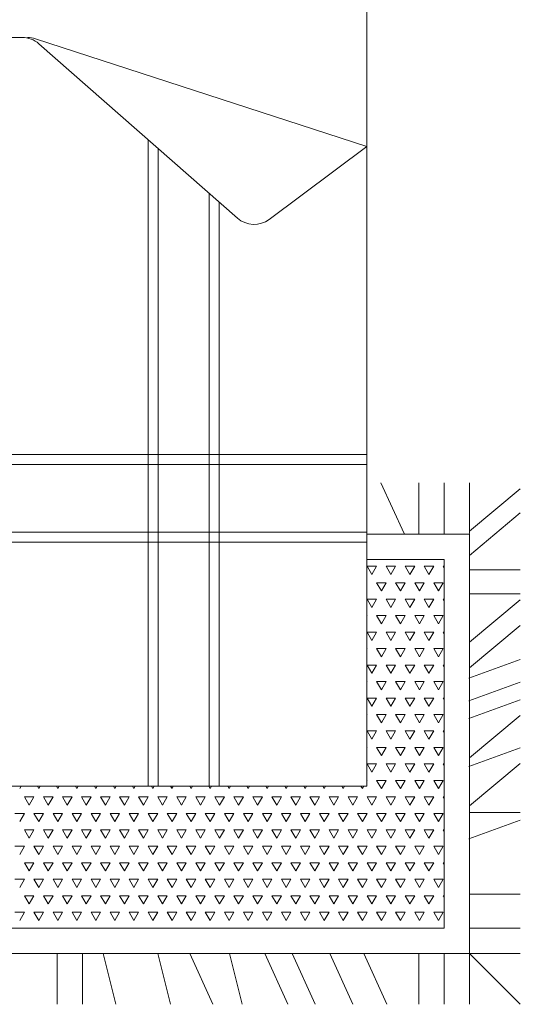
# Model space of a CAD drawing. Units: millimetres. Extents: x 225995 to 227247, y 225507 to 226008.
# Tile 7 of 23: x 226461 to 226503, y 225786 to 225867. Entities that reach past the tile are written whole.
import ezdxf

# ---------------------------------------------------------------- set-up
doc = ezdxf.new("R2010")
doc.units = ezdxf.units.MM
doc.layers.add('A-FURN', color=9, linetype='Continuous', lineweight=18)

# ---------------------------------------------------------------- blocks, each defined once
blk = doc.blocks.new('A$C6D2A2628')
for p, q in [((1.791, 2.4297), (1.791, 0.4297)), ((0.9515, 1.9058), (1.1116, 1.9058)), ((1.791, 1.6908), (1.138, 1.9034)), ((1.1446, 1.8934), (1.5358, 1.5497)), ((1.3599, 1.7043), (1.3599, 0.4297)), ((1.5987, 1.5472), (1.791, 1.6908)), ((1.3799, 1.6867), (1.3799, 0.4297)), ((1.4799, 1.5988), (1.4799, 0.4297)), ((1.4999, 1.5812), (1.4999, 0.4297)), ((0.291, 1.0837), (1.791, 1.0837)), ((0.291, 1.0637), (1.791, 1.0637)), ((1.8187, 1.0278), (1.8641, 0.9278)), ((1.8932, 1.0278), (1.8932, 0.9278)), ((1.9432, 1.0278), (1.9432, 0.9278)), ((1.9932, 1.0278), (1.9932, 0.9278)), ((1.9932, 0.9324), (2.0932, 1.016)), ((1.9932, 0.8849), (2.0932, 0.9685)), ((0.291, 0.9307), (1.791, 0.9307)), ((1.9932, 0.9267), (1.791, 0.9267)), ((1.9932, 0.1), (1.9932, 0.9267)), ((0.291, 0.9107), (1.791, 0.9107)), ((1.9432, 0.8767), (1.791, 0.8767)), ((1.9432, 0.15), (1.9432, 0.8767)), ((1.8007, 0.8473), (1.7913, 0.8636)), ((1.7913, 0.8636), (1.8101, 0.8636)), ((1.8007, 0.8473), (1.8101, 0.8636)), ((1.8382, 0.8473), (1.8288, 0.8636)), ((1.8288, 0.8636), (1.8476, 0.8636)), ((1.8382, 0.8473), (1.8476, 0.8636)), ((1.8757, 0.8473), (1.8663, 0.8636)), ((1.8663, 0.8636), (1.8851, 0.8636)), ((1.8757, 0.8473), (1.8851, 0.8636)), ((1.9132, 0.8473), (1.9038, 0.8636)), ((1.9038, 0.8636), (1.9226, 0.8636)), ((1.9132, 0.8473), (1.9226, 0.8636)), ((1.9432, 0.8604), (1.9413, 0.8636)), ((1.9413, 0.8636), (1.9432, 0.8636)), ((1.9932, 0.8564), (2.0932, 0.8564)), ((1.791, 0.8305), (1.7913, 0.8311)), ((1.791, 0.8311), (1.7913, 0.8311)), ((1.8195, 0.8148), (1.8101, 0.8311)), ((1.8101, 0.8311), (1.8288, 0.8311)), ((1.8195, 0.8148), (1.8288, 0.8311)), ((1.857, 0.8148), (1.8476, 0.8311)), ((1.8476, 0.8311), (1.8663, 0.8311)), ((1.857, 0.8148), (1.8663, 0.8311)), ((1.8945, 0.8148), (1.8851, 0.8311)), ((1.8851, 0.8311), (1.9038, 0.8311)), ((1.8945, 0.8148), (1.9038, 0.8311)), ((1.932, 0.8148), (1.9226, 0.8311)), ((1.9226, 0.8311), (1.9413, 0.8311)), ((1.932, 0.8148), (1.9413, 0.8311)), ((1.8007, 0.7824), (1.7913, 0.7986)), ((1.7913, 0.7986), (1.8101, 0.7986)), ((1.8007, 0.7824), (1.8101, 0.7986)), ((1.8382, 0.7824), (1.8288, 0.7986)), ((1.8288, 0.7986), (1.8476, 0.7986)), ((1.8382, 0.7824), (1.8476, 0.7986)), ((1.8757, 0.7824), (1.8663, 0.7986)), ((1.8663, 0.7986), (1.8851, 0.7986)), ((1.8757, 0.7824), (1.8851, 0.7986)), ((1.9132, 0.7824), (1.9038, 0.7986)), ((1.9038, 0.7986), (1.9226, 0.7986)), ((1.9132, 0.7824), (1.9226, 0.7986)), ((1.9432, 0.7955), (1.9413, 0.7986)), ((1.9413, 0.7986), (1.9432, 0.7986)), ((1.9932, 0.8089), (2.0932, 0.8089)), ((1.9932, 0.7139), (2.0932, 0.7975)), ((1.791, 0.7655), (1.7913, 0.7661)), ((1.791, 0.7661), (1.7913, 0.7661)), ((1.8195, 0.7499), (1.8101, 0.7661)), ((1.8101, 0.7661), (1.8288, 0.7661)), ((1.8195, 0.7499), (1.8288, 0.7661)), ((1.857, 0.7499), (1.8476, 0.7661)), ((1.8476, 0.7661), (1.8663, 0.7661)), ((1.857, 0.7499), (1.8663, 0.7661)), ((1.8945, 0.7499), (1.8851, 0.7661)), ((1.8851, 0.7661), (1.9038, 0.7661)), ((1.8945, 0.7499), (1.9038, 0.7661)), ((1.932, 0.7499), (1.9226, 0.7661)), ((1.9226, 0.7661), (1.9413, 0.7661)), ((1.932, 0.7499), (1.9413, 0.7661)), ((1.9932, 0.6633), (2.0932, 0.7469)), ((1.8007, 0.7174), (1.7913, 0.7337)), ((1.7913, 0.7337), (1.8101, 0.7337)), ((1.8007, 0.7174), (1.8101, 0.7337)), ((1.8382, 0.7174), (1.8288, 0.7337)), ((1.8288, 0.7337), (1.8476, 0.7337)), ((1.8382, 0.7174), (1.8476, 0.7337)), ((1.8757, 0.7174), (1.8663, 0.7337)), ((1.8663, 0.7337), (1.8851, 0.7337)), ((1.8757, 0.7174), (1.8851, 0.7337)), ((1.9132, 0.7174), (1.9038, 0.7337)), ((1.9038, 0.7337), (1.9226, 0.7337)), ((1.9132, 0.7174), (1.9226, 0.7337)), ((1.9432, 0.7305), (1.9413, 0.7337)), ((1.9413, 0.7337), (1.9432, 0.7337)), ((1.791, 0.7006), (1.7913, 0.7012)), ((1.791, 0.7012), (1.7913, 0.7012)), ((1.8195, 0.6849), (1.8101, 0.7012)), ((1.8101, 0.7012), (1.8288, 0.7012)), ((1.8195, 0.6849), (1.8288, 0.7012)), ((1.857, 0.6849), (1.8476, 0.7012)), ((1.8476, 0.7012), (1.8663, 0.7012)), ((1.857, 0.6849), (1.8663, 0.7012)), ((1.8945, 0.6849), (1.8851, 0.7012)), ((1.8851, 0.7012), (1.9038, 0.7012)), ((1.8945, 0.6849), (1.9038, 0.7012)), ((1.932, 0.6849), (1.9226, 0.7012)), ((1.9226, 0.7012), (1.9413, 0.7012)), ((1.932, 0.6849), (1.9413, 0.7012)), ((1.9917, 0.6428), (2.0932, 0.6794)), ((1.8007, 0.6525), (1.7913, 0.6687)), ((1.7913, 0.6687), (1.8101, 0.6687)), ((1.8007, 0.6525), (1.8101, 0.6687)), ((1.8382, 0.6525), (1.8288, 0.6687)), ((1.8288, 0.6687), (1.8476, 0.6687)), ((1.8382, 0.6525), (1.8476, 0.6687)), ((1.8757, 0.6525), (1.8663, 0.6687)), ((1.8663, 0.6687), (1.8851, 0.6687)), ((1.8757, 0.6525), (1.8851, 0.6687)), ((1.9132, 0.6525), (1.9038, 0.6687)), ((1.9038, 0.6687), (1.9226, 0.6687)), ((1.9132, 0.6525), (1.9226, 0.6687)), ((1.9432, 0.6655), (1.9413, 0.6687)), ((1.9413, 0.6687), (1.9432, 0.6687)), ((1.791, 0.6356), (1.7913, 0.6362)), ((1.791, 0.6362), (1.7913, 0.6362)), ((1.8195, 0.62), (1.8101, 0.6362)), ((1.8101, 0.6362), (1.8288, 0.6362)), ((1.8195, 0.62), (1.8288, 0.6362)), ((1.857, 0.62), (1.8476, 0.6362)), ((1.8476, 0.6362), (1.8663, 0.6362)), ((1.857, 0.62), (1.8663, 0.6362)), ((1.8945, 0.62), (1.8851, 0.6362)), ((1.8851, 0.6362), (1.9038, 0.6362)), ((1.8945, 0.62), (1.9038, 0.6362)), ((1.932, 0.62), (1.9226, 0.6362)), ((1.9226, 0.6362), (1.9413, 0.6362)), ((1.932, 0.62), (1.9413, 0.6362)), ((1.9917, 0.5984), (2.0932, 0.6351)), ((1.8007, 0.5875), (1.7913, 0.6037)), ((1.7913, 0.6037), (1.8101, 0.6037)), ((1.8007, 0.5875), (1.8101, 0.6037)), ((1.8382, 0.5875), (1.8288, 0.6037)), ((1.8288, 0.6037), (1.8476, 0.6037)), ((1.8382, 0.5875), (1.8476, 0.6037)), ((1.8757, 0.5875), (1.8663, 0.6037)), ((1.8663, 0.6037), (1.8851, 0.6037)), ((1.8757, 0.5875), (1.8851, 0.6037)), ((1.9132, 0.5875), (1.9038, 0.6037)), ((1.9038, 0.6037), (1.9226, 0.6037)), ((1.9132, 0.5875), (1.9226, 0.6037)), ((1.9432, 0.6006), (1.9413, 0.6037)), ((1.9413, 0.6037), (1.9432, 0.6037)), ((1.9917, 0.5636), (2.0932, 0.6003)), ((1.791, 0.5707), (1.7913, 0.5713)), ((1.791, 0.5713), (1.7913, 0.5713)), ((1.8195, 0.555), (1.8101, 0.5713)), ((1.8101, 0.5713), (1.8288, 0.5713)), ((1.8195, 0.555), (1.8288, 0.5713)), ((1.857, 0.555), (1.8476, 0.5713)), ((1.8476, 0.5713), (1.8663, 0.5713)), ((1.857, 0.555), (1.8663, 0.5713)), ((1.8945, 0.555), (1.8851, 0.5713)), ((1.8851, 0.5713), (1.9038, 0.5713)), ((1.8945, 0.555), (1.9038, 0.5713)), ((1.932, 0.555), (1.9226, 0.5713)), ((1.9226, 0.5713), (1.9413, 0.5713)), ((1.932, 0.555), (1.9413, 0.5713)), ((1.9932, 0.4859), (2.0932, 0.5695)), ((1.8007, 0.5226), (1.7913, 0.5388)), ((1.7913, 0.5388), (1.8101, 0.5388)), ((1.8007, 0.5226), (1.8101, 0.5388)), ((1.8382, 0.5226), (1.8288, 0.5388)), ((1.8288, 0.5388), (1.8476, 0.5388)), ((1.8382, 0.5226), (1.8476, 0.5388)), ((1.8757, 0.5226), (1.8663, 0.5388)), ((1.8663, 0.5388), (1.8851, 0.5388)), ((1.8757, 0.5226), (1.8851, 0.5388)), ((1.9132, 0.5226), (1.9038, 0.5388)), ((1.9038, 0.5388), (1.9226, 0.5388)), ((1.9132, 0.5226), (1.9226, 0.5388)), ((1.9432, 0.5356), (1.9413, 0.5388)), ((1.9413, 0.5388), (1.9432, 0.5388)), ((1.791, 0.5057), (1.7913, 0.5063)), ((1.791, 0.5063), (1.7913, 0.5063)), ((1.8195, 0.4901), (1.8101, 0.5063)), ((1.8101, 0.5063), (1.8288, 0.5063)), ((1.8195, 0.4901), (1.8288, 0.5063)), ((1.857, 0.4901), (1.8476, 0.5063)), ((1.8476, 0.5063), (1.8663, 0.5063)), ((1.857, 0.4901), (1.8663, 0.5063)), ((1.8945, 0.4901), (1.8851, 0.5063)), ((1.8851, 0.5063), (1.9038, 0.5063)), ((1.8945, 0.4901), (1.9038, 0.5063)), ((1.932, 0.4901), (1.9226, 0.5063)), ((1.9226, 0.5063), (1.9413, 0.5063)), ((1.932, 0.4901), (1.9413, 0.5063)), ((1.9917, 0.4686), (2.0932, 0.5053)), ((1.8007, 0.4576), (1.7913, 0.4738)), ((1.7913, 0.4738), (1.8101, 0.4738)), ((1.8007, 0.4576), (1.8101, 0.4738)), ((1.8382, 0.4576), (1.8288, 0.4738)), ((1.8288, 0.4738), (1.8476, 0.4738)), ((1.8382, 0.4576), (1.8476, 0.4738)), ((1.8757, 0.4576), (1.8663, 0.4738)), ((1.8663, 0.4738), (1.8851, 0.4738)), ((1.8757, 0.4576), (1.8851, 0.4738)), ((1.9132, 0.4576), (1.9038, 0.4738)), ((1.9038, 0.4738), (1.9226, 0.4738)), ((1.9132, 0.4576), (1.9226, 0.4738)), ((1.9432, 0.4707), (1.9413, 0.4738)), ((1.9413, 0.4738), (1.9432, 0.4738)), ((1.9932, 0.3909), (2.0932, 0.4745)), ((1.791, 0.4297), (0.291, 0.4297)), ((1.107, 0.4251), (1.1096, 0.4297)), ((1.1445, 0.4251), (1.1418, 0.4297)), ((1.1445, 0.4251), (1.1471, 0.4297)), ((1.182, 0.4251), (1.1793, 0.4297)), ((1.182, 0.4251), (1.1846, 0.4297)), ((1.2195, 0.4251), (1.2168, 0.4297)), ((1.2195, 0.4251), (1.2221, 0.4297)), ((1.257, 0.4251), (1.2543, 0.4297)), ((1.257, 0.4251), (1.2596, 0.4297)), ((1.2945, 0.4251), (1.2918, 0.4297)), ((1.2945, 0.4251), (1.2971, 0.4297)), ((1.332, 0.4251), (1.3293, 0.4297)), ((1.332, 0.4251), (1.3346, 0.4297)), ((1.3695, 0.4251), (1.3668, 0.4297)), ((1.3695, 0.4251), (1.3721, 0.4297)), ((1.407, 0.4251), (1.4043, 0.4297)), ((1.407, 0.4251), (1.4096, 0.4297)), ((1.4445, 0.4251), (1.4418, 0.4297)), ((1.4445, 0.4251), (1.4471, 0.4297)), ((1.482, 0.4251), (1.4793, 0.4297)), ((1.482, 0.4251), (1.4846, 0.4297)), ((1.5195, 0.4251), (1.5168, 0.4297)), ((1.5195, 0.4251), (1.5221, 0.4297)), ((1.557, 0.4251), (1.5543, 0.4297)), ((1.557, 0.4251), (1.5596, 0.4297)), ((1.5945, 0.4251), (1.5918, 0.4297)), ((1.5945, 0.4251), (1.5971, 0.4297)), ((1.632, 0.4251), (1.6293, 0.4297)), ((1.632, 0.4251), (1.6346, 0.4297)), ((1.6695, 0.4251), (1.6668, 0.4297)), ((1.6695, 0.4251), (1.6721, 0.4297)), ((1.707, 0.4251), (1.7043, 0.4297)), ((1.707, 0.4251), (1.7096, 0.4297)), ((1.7445, 0.4251), (1.7418, 0.4297)), ((1.7445, 0.4251), (1.7471, 0.4297)), ((1.782, 0.4251), (1.7793, 0.4297)), ((1.782, 0.4251), (1.7846, 0.4297)), ((1.791, 0.4408), (1.7913, 0.4414)), ((1.791, 0.4414), (1.7913, 0.4414)), ((1.8195, 0.4251), (1.8101, 0.4414)), ((1.8101, 0.4414), (1.8288, 0.4414)), ((1.8195, 0.4251), (1.8288, 0.4414)), ((1.857, 0.4251), (1.8476, 0.4414)), ((1.8476, 0.4414), (1.8663, 0.4414)), ((1.857, 0.4251), (1.8663, 0.4414)), ((1.8945, 0.4251), (1.8851, 0.4414)), ((1.8851, 0.4414), (1.9038, 0.4414)), ((1.8945, 0.4251), (1.9038, 0.4414)), ((1.932, 0.4251), (1.9226, 0.4414)), ((1.9226, 0.4414), (1.9413, 0.4414)), ((1.932, 0.4251), (1.9413, 0.4414)), ((1.1257, 0.3927), (1.1163, 0.4089)), ((1.1163, 0.4089), (1.1351, 0.4089)), ((1.1257, 0.3927), (1.1351, 0.4089)), ((1.1632, 0.3927), (1.1538, 0.4089)), ((1.1538, 0.4089), (1.1726, 0.4089)), ((1.1632, 0.3927), (1.1726, 0.4089)), ((1.2007, 0.3927), (1.1913, 0.4089)), ((1.1913, 0.4089), (1.2101, 0.4089)), ((1.2007, 0.3927), (1.2101, 0.4089)), ((1.2382, 0.3927), (1.2288, 0.4089)), ((1.2288, 0.4089), (1.2476, 0.4089)), ((1.2382, 0.3927), (1.2476, 0.4089)), ((1.2757, 0.3927), (1.2663, 0.4089)), ((1.2663, 0.4089), (1.2851, 0.4089)), ((1.2757, 0.3927), (1.2851, 0.4089)), ((1.3132, 0.3927), (1.3038, 0.4089)), ((1.3038, 0.4089), (1.3226, 0.4089)), ((1.3132, 0.3927), (1.3226, 0.4089)), ((1.3507, 0.3927), (1.3413, 0.4089)), ((1.3413, 0.4089), (1.3601, 0.4089)), ((1.3507, 0.3927), (1.3601, 0.4089)), ((1.3882, 0.3927), (1.3788, 0.4089)), ((1.3788, 0.4089), (1.3976, 0.4089)), ((1.3882, 0.3927), (1.3976, 0.4089)), ((1.4257, 0.3927), (1.4163, 0.4089)), ((1.4163, 0.4089), (1.4351, 0.4089)), ((1.4257, 0.3927), (1.4351, 0.4089)), ((1.4632, 0.3927), (1.4538, 0.4089)), ((1.4538, 0.4089), (1.4726, 0.4089)), ((1.4632, 0.3927), (1.4726, 0.4089)), ((1.5007, 0.3927), (1.4913, 0.4089)), ((1.4913, 0.4089), (1.5101, 0.4089)), ((1.5007, 0.3927), (1.5101, 0.4089)), ((1.5382, 0.3927), (1.5288, 0.4089)), ((1.5288, 0.4089), (1.5476, 0.4089)), ((1.5382, 0.3927), (1.5476, 0.4089)), ((1.5757, 0.3927), (1.5663, 0.4089)), ((1.5663, 0.4089), (1.5851, 0.4089)), ((1.5757, 0.3927), (1.5851, 0.4089)), ((1.6132, 0.3927), (1.6038, 0.4089)), ((1.6038, 0.4089), (1.6226, 0.4089)), ((1.6132, 0.3927), (1.6226, 0.4089)), ((1.6507, 0.3927), (1.6413, 0.4089)), ((1.6413, 0.4089), (1.6601, 0.4089)), ((1.6507, 0.3927), (1.6601, 0.4089)), ((1.6882, 0.3927), (1.6788, 0.4089)), ((1.6788, 0.4089), (1.6976, 0.4089)), ((1.6882, 0.3927), (1.6976, 0.4089)), ((1.7257, 0.3927), (1.7163, 0.4089)), ((1.7163, 0.4089), (1.7351, 0.4089)), ((1.7257, 0.3927), (1.7351, 0.4089)), ((1.7632, 0.3927), (1.7538, 0.4089)), ((1.7538, 0.4089), (1.7726, 0.4089)), ((1.7632, 0.3927), (1.7726, 0.4089)), ((1.8007, 0.3927), (1.7913, 0.4089)), ((1.7913, 0.4089), (1.8101, 0.4089)), ((1.8007, 0.3927), (1.8101, 0.4089)), ((1.8382, 0.3927), (1.8288, 0.4089)), ((1.8288, 0.4089), (1.8476, 0.4089)), ((1.8382, 0.3927), (1.8476, 0.4089)), ((1.8757, 0.3927), (1.8663, 0.4089)), ((1.8663, 0.4089), (1.8851, 0.4089)), ((1.8757, 0.3927), (1.8851, 0.4089)), ((1.9132, 0.3927), (1.9038, 0.4089)), ((1.9038, 0.4089), (1.9226, 0.4089)), ((1.9132, 0.3927), (1.9226, 0.4089)), ((1.9432, 0.4057), (1.9413, 0.4089)), ((1.9413, 0.4089), (1.9432, 0.4089)), ((1.0976, 0.3764), (1.1163, 0.3764)), ((1.107, 0.3602), (1.1163, 0.3764)), ((1.1445, 0.3602), (1.1351, 0.3764)), ((1.1351, 0.3764), (1.1538, 0.3764)), ((1.1445, 0.3602), (1.1538, 0.3764)), ((1.182, 0.3602), (1.1726, 0.3764)), ((1.1726, 0.3764), (1.1913, 0.3764)), ((1.182, 0.3602), (1.1913, 0.3764)), ((1.2195, 0.3602), (1.2101, 0.3764)), ((1.2101, 0.3764), (1.2288, 0.3764)), ((1.2195, 0.3602), (1.2288, 0.3764)), ((1.257, 0.3602), (1.2476, 0.3764)), ((1.2476, 0.3764), (1.2663, 0.3764)), ((1.257, 0.3602), (1.2663, 0.3764)), ((1.2945, 0.3602), (1.2851, 0.3764)), ((1.2851, 0.3764), (1.3038, 0.3764)), ((1.2945, 0.3602), (1.3038, 0.3764)), ((1.332, 0.3602), (1.3226, 0.3764)), ((1.3226, 0.3764), (1.3413, 0.3764)), ((1.332, 0.3602), (1.3413, 0.3764)), ((1.3695, 0.3602), (1.3601, 0.3764)), ((1.3601, 0.3764), (1.3788, 0.3764)), ((1.3695, 0.3602), (1.3788, 0.3764)), ((1.407, 0.3602), (1.3976, 0.3764)), ((1.3976, 0.3764), (1.4163, 0.3764)), ((1.407, 0.3602), (1.4163, 0.3764)), ((1.4445, 0.3602), (1.4351, 0.3764)), ((1.4351, 0.3764), (1.4538, 0.3764)), ((1.4445, 0.3602), (1.4538, 0.3764)), ((1.482, 0.3602), (1.4726, 0.3764)), ((1.4726, 0.3764), (1.4913, 0.3764)), ((1.482, 0.3602), (1.4913, 0.3764)), ((1.5195, 0.3602), (1.5101, 0.3764)), ((1.5101, 0.3764), (1.5288, 0.3764)), ((1.5195, 0.3602), (1.5288, 0.3764)), ((1.557, 0.3602), (1.5476, 0.3764)), ((1.5476, 0.3764), (1.5663, 0.3764)), ((1.557, 0.3602), (1.5663, 0.3764)), ((1.5945, 0.3602), (1.5851, 0.3764)), ((1.5851, 0.3764), (1.6038, 0.3764)), ((1.5945, 0.3602), (1.6038, 0.3764)), ((1.632, 0.3602), (1.6226, 0.3764)), ((1.6226, 0.3764), (1.6413, 0.3764)), ((1.632, 0.3602), (1.6413, 0.3764)), ((1.6695, 0.3602), (1.6601, 0.3764)), ((1.6601, 0.3764), (1.6788, 0.3764)), ((1.6695, 0.3602), (1.6788, 0.3764)), ((1.707, 0.3602), (1.6976, 0.3764)), ((1.6976, 0.3764), (1.7163, 0.3764)), ((1.707, 0.3602), (1.7163, 0.3764)), ((1.7445, 0.3602), (1.7351, 0.3764)), ((1.7351, 0.3764), (1.7538, 0.3764)), ((1.7445, 0.3602), (1.7538, 0.3764)), ((1.782, 0.3602), (1.7726, 0.3764)), ((1.7726, 0.3764), (1.7913, 0.3764)), ((1.782, 0.3602), (1.7913, 0.3764)), ((1.8195, 0.3602), (1.8101, 0.3764)), ((1.8101, 0.3764), (1.8288, 0.3764)), ((1.8195, 0.3602), (1.8288, 0.3764)), ((1.857, 0.3602), (1.8476, 0.3764)), ((1.8476, 0.3764), (1.8663, 0.3764)), ((1.857, 0.3602), (1.8663, 0.3764)), ((1.8945, 0.3602), (1.8851, 0.3764)), ((1.8851, 0.3764), (1.9038, 0.3764)), ((1.8945, 0.3602), (1.9038, 0.3764)), ((1.932, 0.3602), (1.9226, 0.3764)), ((1.9226, 0.3764), (1.9413, 0.3764)), ((1.932, 0.3602), (1.9413, 0.3764)), ((1.9932, 0.3783), (2.0932, 0.3783)), ((1.9917, 0.3261), (2.0932, 0.3628)), ((1.1257, 0.3277), (1.1163, 0.3439)), ((1.1163, 0.3439), (1.1351, 0.3439)), ((1.1257, 0.3277), (1.1351, 0.3439)), ((1.1632, 0.3277), (1.1538, 0.3439)), ((1.1538, 0.3439), (1.1726, 0.3439)), ((1.1632, 0.3277), (1.1726, 0.3439)), ((1.2007, 0.3277), (1.1913, 0.3439)), ((1.1913, 0.3439), (1.2101, 0.3439)), ((1.2007, 0.3277), (1.2101, 0.3439)), ((1.2382, 0.3277), (1.2288, 0.3439)), ((1.2288, 0.3439), (1.2476, 0.3439)), ((1.2382, 0.3277), (1.2476, 0.3439)), ((1.2757, 0.3277), (1.2663, 0.3439)), ((1.2663, 0.3439), (1.2851, 0.3439)), ((1.2757, 0.3277), (1.2851, 0.3439)), ((1.3132, 0.3277), (1.3038, 0.3439)), ((1.3038, 0.3439), (1.3226, 0.3439)), ((1.3132, 0.3277), (1.3226, 0.3439)), ((1.3507, 0.3277), (1.3413, 0.3439)), ((1.3413, 0.3439), (1.3601, 0.3439)), ((1.3507, 0.3277), (1.3601, 0.3439)), ((1.3882, 0.3277), (1.3788, 0.3439)), ((1.3788, 0.3439), (1.3976, 0.3439)), ((1.3882, 0.3277), (1.3976, 0.3439)), ((1.4257, 0.3277), (1.4163, 0.3439)), ((1.4163, 0.3439), (1.4351, 0.3439)), ((1.4257, 0.3277), (1.4351, 0.3439)), ((1.4632, 0.3277), (1.4538, 0.3439)), ((1.4538, 0.3439), (1.4726, 0.3439)), ((1.4632, 0.3277), (1.4726, 0.3439)), ((1.5007, 0.3277), (1.4913, 0.3439)), ((1.4913, 0.3439), (1.5101, 0.3439)), ((1.5007, 0.3277), (1.5101, 0.3439)), ((1.5382, 0.3277), (1.5288, 0.3439)), ((1.5288, 0.3439), (1.5476, 0.3439)), ((1.5382, 0.3277), (1.5476, 0.3439)), ((1.5757, 0.3277), (1.5663, 0.3439)), ((1.5663, 0.3439), (1.5851, 0.3439)), ((1.5757, 0.3277), (1.5851, 0.3439)), ((1.6132, 0.3277), (1.6038, 0.3439)), ((1.6038, 0.3439), (1.6226, 0.3439)), ((1.6132, 0.3277), (1.6226, 0.3439)), ((1.6507, 0.3277), (1.6413, 0.3439)), ((1.6413, 0.3439), (1.6601, 0.3439)), ((1.6507, 0.3277), (1.6601, 0.3439)), ((1.6882, 0.3277), (1.6788, 0.3439)), ((1.6788, 0.3439), (1.6976, 0.3439)), ((1.6882, 0.3277), (1.6976, 0.3439)), ((1.7257, 0.3277), (1.7163, 0.3439)), ((1.7163, 0.3439), (1.7351, 0.3439)), ((1.7257, 0.3277), (1.7351, 0.3439)), ((1.7632, 0.3277), (1.7538, 0.3439)), ((1.7538, 0.3439), (1.7726, 0.3439)), ((1.7632, 0.3277), (1.7726, 0.3439)), ((1.8007, 0.3277), (1.7913, 0.3439)), ((1.7913, 0.3439), (1.8101, 0.3439)), ((1.8007, 0.3277), (1.8101, 0.3439)), ((1.8382, 0.3277), (1.8288, 0.3439)), ((1.8288, 0.3439), (1.8476, 0.3439)), ((1.8382, 0.3277), (1.8476, 0.3439)), ((1.8757, 0.3277), (1.8663, 0.3439)), ((1.8663, 0.3439), (1.8851, 0.3439)), ((1.8757, 0.3277), (1.8851, 0.3439)), ((1.9132, 0.3277), (1.9038, 0.3439)), ((1.9038, 0.3439), (1.9226, 0.3439)), ((1.9132, 0.3277), (1.9226, 0.3439)), ((1.9432, 0.3408), (1.9413, 0.3439)), ((1.9413, 0.3439), (1.9432, 0.3439)), ((1.0976, 0.3115), (1.1163, 0.3115)), ((1.107, 0.2952), (1.1163, 0.3115)), ((1.1445, 0.2952), (1.1351, 0.3115)), ((1.1351, 0.3115), (1.1538, 0.3115)), ((1.1445, 0.2952), (1.1538, 0.3115)), ((1.182, 0.2952), (1.1726, 0.3115)), ((1.1726, 0.3115), (1.1913, 0.3115)), ((1.182, 0.2952), (1.1913, 0.3115)), ((1.2195, 0.2952), (1.2101, 0.3115)), ((1.2101, 0.3115), (1.2288, 0.3115)), ((1.2195, 0.2952), (1.2288, 0.3115)), ((1.257, 0.2952), (1.2476, 0.3115)), ((1.2476, 0.3115), (1.2663, 0.3115)), ((1.257, 0.2952), (1.2663, 0.3115)), ((1.2945, 0.2952), (1.2851, 0.3115)), ((1.2851, 0.3115), (1.3038, 0.3115)), ((1.2945, 0.2952), (1.3038, 0.3115)), ((1.332, 0.2952), (1.3226, 0.3115)), ((1.3226, 0.3115), (1.3413, 0.3115)), ((1.332, 0.2952), (1.3413, 0.3115)), ((1.3695, 0.2952), (1.3601, 0.3115)), ((1.3601, 0.3115), (1.3788, 0.3115)), ((1.3695, 0.2952), (1.3788, 0.3115)), ((1.407, 0.2952), (1.3976, 0.3115)), ((1.3976, 0.3115), (1.4163, 0.3115)), ((1.407, 0.2952), (1.4163, 0.3115)), ((1.4445, 0.2952), (1.4351, 0.3115)), ((1.4351, 0.3115), (1.4538, 0.3115)), ((1.4445, 0.2952), (1.4538, 0.3115)), ((1.482, 0.2952), (1.4726, 0.3115)), ((1.4726, 0.3115), (1.4913, 0.3115)), ((1.482, 0.2952), (1.4913, 0.3115)), ((1.5195, 0.2952), (1.5101, 0.3115)), ((1.5101, 0.3115), (1.5288, 0.3115)), ((1.5195, 0.2952), (1.5288, 0.3115)), ((1.557, 0.2952), (1.5476, 0.3115)), ((1.5476, 0.3115), (1.5663, 0.3115)), ((1.557, 0.2952), (1.5663, 0.3115)), ((1.5945, 0.2952), (1.5851, 0.3115)), ((1.5851, 0.3115), (1.6038, 0.3115)), ((1.5945, 0.2952), (1.6038, 0.3115)), ((1.632, 0.2952), (1.6226, 0.3115)), ((1.6226, 0.3115), (1.6413, 0.3115)), ((1.632, 0.2952), (1.6413, 0.3115)), ((1.6695, 0.2952), (1.6601, 0.3115)), ((1.6601, 0.3115), (1.6788, 0.3115)), ((1.6695, 0.2952), (1.6788, 0.3115)), ((1.707, 0.2952), (1.6976, 0.3115)), ((1.6976, 0.3115), (1.7163, 0.3115)), ((1.707, 0.2952), (1.7163, 0.3115)), ((1.7445, 0.2952), (1.7351, 0.3115)), ((1.7351, 0.3115), (1.7538, 0.3115)), ((1.7445, 0.2952), (1.7538, 0.3115)), ((1.782, 0.2952), (1.7726, 0.3115)), ((1.7726, 0.3115), (1.7913, 0.3115)), ((1.782, 0.2952), (1.7913, 0.3115)), ((1.8195, 0.2952), (1.8101, 0.3115)), ((1.8101, 0.3115), (1.8288, 0.3115)), ((1.8195, 0.2952), (1.8288, 0.3115)), ((1.857, 0.2952), (1.8476, 0.3115)), ((1.8476, 0.3115), (1.8663, 0.3115)), ((1.857, 0.2952), (1.8663, 0.3115)), ((1.8945, 0.2952), (1.8851, 0.3115)), ((1.8851, 0.3115), (1.9038, 0.3115)), ((1.8945, 0.2952), (1.9038, 0.3115)), ((1.932, 0.2952), (1.9226, 0.3115)), ((1.9226, 0.3115), (1.9413, 0.3115)), ((1.932, 0.2952), (1.9413, 0.3115)), ((1.1257, 0.2628), (1.1163, 0.279)), ((1.1163, 0.279), (1.1351, 0.279)), ((1.1257, 0.2628), (1.1351, 0.279)), ((1.1632, 0.2628), (1.1538, 0.279)), ((1.1538, 0.279), (1.1726, 0.279)), ((1.1632, 0.2628), (1.1726, 0.279)), ((1.2007, 0.2628), (1.1913, 0.279)), ((1.1913, 0.279), (1.2101, 0.279)), ((1.2007, 0.2628), (1.2101, 0.279)), ((1.2382, 0.2628), (1.2288, 0.279)), ((1.2288, 0.279), (1.2476, 0.279)), ((1.2382, 0.2628), (1.2476, 0.279)), ((1.2757, 0.2628), (1.2663, 0.279)), ((1.2663, 0.279), (1.2851, 0.279)), ((1.2757, 0.2628), (1.2851, 0.279)), ((1.3132, 0.2628), (1.3038, 0.279)), ((1.3038, 0.279), (1.3226, 0.279)), ((1.3132, 0.2628), (1.3226, 0.279)), ((1.3507, 0.2628), (1.3413, 0.279)), ((1.3413, 0.279), (1.3601, 0.279)), ((1.3507, 0.2628), (1.3601, 0.279)), ((1.3882, 0.2628), (1.3788, 0.279)), ((1.3788, 0.279), (1.3976, 0.279)), ((1.3882, 0.2628), (1.3976, 0.279)), ((1.4257, 0.2628), (1.4163, 0.279)), ((1.4163, 0.279), (1.4351, 0.279)), ((1.4257, 0.2628), (1.4351, 0.279)), ((1.4632, 0.2628), (1.4538, 0.279)), ((1.4538, 0.279), (1.4726, 0.279)), ((1.4632, 0.2628), (1.4726, 0.279)), ((1.5007, 0.2628), (1.4913, 0.279)), ((1.4913, 0.279), (1.5101, 0.279)), ((1.5007, 0.2628), (1.5101, 0.279)), ((1.5382, 0.2628), (1.5288, 0.279)), ((1.5288, 0.279), (1.5476, 0.279)), ((1.5382, 0.2628), (1.5476, 0.279)), ((1.5757, 0.2628), (1.5663, 0.279)), ((1.5663, 0.279), (1.5851, 0.279)), ((1.5757, 0.2628), (1.5851, 0.279)), ((1.6132, 0.2628), (1.6038, 0.279)), ((1.6038, 0.279), (1.6226, 0.279)), ((1.6132, 0.2628), (1.6226, 0.279)), ((1.6507, 0.2628), (1.6413, 0.279)), ((1.6413, 0.279), (1.6601, 0.279)), ((1.6507, 0.2628), (1.6601, 0.279)), ((1.6882, 0.2628), (1.6788, 0.279)), ((1.6788, 0.279), (1.6976, 0.279)), ((1.6882, 0.2628), (1.6976, 0.279)), ((1.7257, 0.2628), (1.7163, 0.279)), ((1.7163, 0.279), (1.7351, 0.279)), ((1.7257, 0.2628), (1.7351, 0.279)), ((1.7632, 0.2628), (1.7538, 0.279)), ((1.7538, 0.279), (1.7726, 0.279)), ((1.7632, 0.2628), (1.7726, 0.279)), ((1.8007, 0.2628), (1.7913, 0.279)), ((1.7913, 0.279), (1.8101, 0.279)), ((1.8007, 0.2628), (1.8101, 0.279)), ((1.8382, 0.2628), (1.8288, 0.279)), ((1.8288, 0.279), (1.8476, 0.279)), ((1.8382, 0.2628), (1.8476, 0.279)), ((1.8757, 0.2628), (1.8663, 0.279)), ((1.8663, 0.279), (1.8851, 0.279)), ((1.8757, 0.2628), (1.8851, 0.279)), ((1.9132, 0.2628), (1.9038, 0.279)), ((1.9038, 0.279), (1.9226, 0.279)), ((1.9132, 0.2628), (1.9226, 0.279)), ((1.9432, 0.2758), (1.9413, 0.279)), ((1.9413, 0.279), (1.9432, 0.279)), ((1.0976, 0.2465), (1.1163, 0.2465)), ((1.107, 0.2303), (1.1163, 0.2465)), ((1.1445, 0.2303), (1.1351, 0.2465)), ((1.1351, 0.2465), (1.1538, 0.2465)), ((1.1445, 0.2303), (1.1538, 0.2465)), ((1.182, 0.2303), (1.1726, 0.2465)), ((1.1726, 0.2465), (1.1913, 0.2465)), ((1.182, 0.2303), (1.1913, 0.2465)), ((1.2195, 0.2303), (1.2101, 0.2465)), ((1.2101, 0.2465), (1.2288, 0.2465)), ((1.2195, 0.2303), (1.2288, 0.2465)), ((1.257, 0.2303), (1.2476, 0.2465)), ((1.2476, 0.2465), (1.2663, 0.2465)), ((1.257, 0.2303), (1.2663, 0.2465)), ((1.2945, 0.2303), (1.2851, 0.2465)), ((1.2851, 0.2465), (1.3038, 0.2465)), ((1.2945, 0.2303), (1.3038, 0.2465)), ((1.332, 0.2303), (1.3226, 0.2465)), ((1.3226, 0.2465), (1.3413, 0.2465)), ((1.332, 0.2303), (1.3413, 0.2465)), ((1.3695, 0.2303), (1.3601, 0.2465)), ((1.3601, 0.2465), (1.3788, 0.2465)), ((1.3695, 0.2303), (1.3788, 0.2465)), ((1.407, 0.2303), (1.3976, 0.2465)), ((1.3976, 0.2465), (1.4163, 0.2465)), ((1.407, 0.2303), (1.4163, 0.2465)), ((1.4445, 0.2303), (1.4351, 0.2465)), ((1.4351, 0.2465), (1.4538, 0.2465)), ((1.4445, 0.2303), (1.4538, 0.2465)), ((1.482, 0.2303), (1.4726, 0.2465)), ((1.4726, 0.2465), (1.4913, 0.2465)), ((1.482, 0.2303), (1.4913, 0.2465)), ((1.5195, 0.2303), (1.5101, 0.2465)), ((1.5101, 0.2465), (1.5288, 0.2465)), ((1.5195, 0.2303), (1.5288, 0.2465)), ((1.557, 0.2303), (1.5476, 0.2465)), ((1.5476, 0.2465), (1.5663, 0.2465)), ((1.557, 0.2303), (1.5663, 0.2465)), ((1.5945, 0.2303), (1.5851, 0.2465)), ((1.5851, 0.2465), (1.6038, 0.2465)), ((1.5945, 0.2303), (1.6038, 0.2465)), ((1.632, 0.2303), (1.6226, 0.2465)), ((1.6226, 0.2465), (1.6413, 0.2465)), ((1.632, 0.2303), (1.6413, 0.2465)), ((1.6695, 0.2303), (1.6601, 0.2465)), ((1.6601, 0.2465), (1.6788, 0.2465)), ((1.6695, 0.2303), (1.6788, 0.2465)), ((1.707, 0.2303), (1.6976, 0.2465)), ((1.6976, 0.2465), (1.7163, 0.2465)), ((1.707, 0.2303), (1.7163, 0.2465)), ((1.7445, 0.2303), (1.7351, 0.2465)), ((1.7351, 0.2465), (1.7538, 0.2465)), ((1.7445, 0.2303), (1.7538, 0.2465)), ((1.782, 0.2303), (1.7726, 0.2465)), ((1.7726, 0.2465), (1.7913, 0.2465)), ((1.782, 0.2303), (1.7913, 0.2465)), ((1.8195, 0.2303), (1.8101, 0.2465)), ((1.8101, 0.2465), (1.8288, 0.2465)), ((1.8195, 0.2303), (1.8288, 0.2465)), ((1.857, 0.2303), (1.8476, 0.2465)), ((1.8476, 0.2465), (1.8663, 0.2465)), ((1.857, 0.2303), (1.8663, 0.2465)), ((1.8945, 0.2303), (1.8851, 0.2465)), ((1.8851, 0.2465), (1.9038, 0.2465)), ((1.8945, 0.2303), (1.9038, 0.2465)), ((1.932, 0.2303), (1.9226, 0.2465)), ((1.9226, 0.2465), (1.9413, 0.2465)), ((1.932, 0.2303), (1.9413, 0.2465)), ((1.1257, 0.1978), (1.1163, 0.214)), ((1.1163, 0.214), (1.1351, 0.214)), ((1.1257, 0.1978), (1.1351, 0.214)), ((1.1632, 0.1978), (1.1538, 0.214)), ((1.1538, 0.214), (1.1726, 0.214)), ((1.1632, 0.1978), (1.1726, 0.214)), ((1.2007, 0.1978), (1.1913, 0.214)), ((1.1913, 0.214), (1.2101, 0.214)), ((1.2007, 0.1978), (1.2101, 0.214)), ((1.2382, 0.1978), (1.2288, 0.214)), ((1.2288, 0.214), (1.2476, 0.214)), ((1.2382, 0.1978), (1.2476, 0.214)), ((1.2757, 0.1978), (1.2663, 0.214)), ((1.2663, 0.214), (1.2851, 0.214)), ((1.2757, 0.1978), (1.2851, 0.214)), ((1.3132, 0.1978), (1.3038, 0.214)), ((1.3038, 0.214), (1.3226, 0.214)), ((1.3132, 0.1978), (1.3226, 0.214)), ((1.3507, 0.1978), (1.3413, 0.214)), ((1.3413, 0.214), (1.3601, 0.214)), ((1.3507, 0.1978), (1.3601, 0.214)), ((1.3882, 0.1978), (1.3788, 0.214)), ((1.3788, 0.214), (1.3976, 0.214)), ((1.3882, 0.1978), (1.3976, 0.214)), ((1.4257, 0.1978), (1.4163, 0.214)), ((1.4163, 0.214), (1.4351, 0.214)), ((1.4257, 0.1978), (1.4351, 0.214)), ((1.4632, 0.1978), (1.4538, 0.214)), ((1.4538, 0.214), (1.4726, 0.214)), ((1.4632, 0.1978), (1.4726, 0.214)), ((1.5007, 0.1978), (1.4913, 0.214)), ((1.4913, 0.214), (1.5101, 0.214)), ((1.5007, 0.1978), (1.5101, 0.214)), ((1.5382, 0.1978), (1.5288, 0.214)), ((1.5288, 0.214), (1.5476, 0.214)), ((1.5382, 0.1978), (1.5476, 0.214)), ((1.5757, 0.1978), (1.5663, 0.214)), ((1.5663, 0.214), (1.5851, 0.214)), ((1.5757, 0.1978), (1.5851, 0.214)), ((1.6132, 0.1978), (1.6038, 0.214)), ((1.6038, 0.214), (1.6226, 0.214)), ((1.6132, 0.1978), (1.6226, 0.214)), ((1.6507, 0.1978), (1.6413, 0.214)), ((1.6413, 0.214), (1.6601, 0.214)), ((1.6507, 0.1978), (1.6601, 0.214)), ((1.6882, 0.1978), (1.6788, 0.214)), ((1.6788, 0.214), (1.6976, 0.214)), ((1.6882, 0.1978), (1.6976, 0.214)), ((1.7257, 0.1978), (1.7163, 0.214)), ((1.7163, 0.214), (1.7351, 0.214)), ((1.7257, 0.1978), (1.7351, 0.214)), ((1.7632, 0.1978), (1.7538, 0.214)), ((1.7538, 0.214), (1.7726, 0.214)), ((1.7632, 0.1978), (1.7726, 0.214)), ((1.8007, 0.1978), (1.7913, 0.214)), ((1.7913, 0.214), (1.8101, 0.214)), ((1.8007, 0.1978), (1.8101, 0.214)), ((1.8382, 0.1978), (1.8288, 0.214)), ((1.8288, 0.214), (1.8476, 0.214)), ((1.8382, 0.1978), (1.8476, 0.214)), ((1.8757, 0.1978), (1.8663, 0.214)), ((1.8663, 0.214), (1.8851, 0.214)), ((1.8757, 0.1978), (1.8851, 0.214)), ((1.9132, 0.1978), (1.9038, 0.214)), ((1.9038, 0.214), (1.9226, 0.214)), ((1.9132, 0.1978), (1.9226, 0.214)), ((1.9432, 0.2109), (1.9413, 0.214)), ((1.9413, 0.214), (1.9432, 0.214)), ((1.9932, 0.2173), (2.0932, 0.2173)), ((1.0976, 0.1816), (1.1163, 0.1816)), ((1.107, 0.1653), (1.1163, 0.1816)), ((1.1445, 0.1653), (1.1351, 0.1816)), ((1.1351, 0.1816), (1.1538, 0.1816)), ((1.1445, 0.1653), (1.1538, 0.1816)), ((1.182, 0.1653), (1.1726, 0.1816)), ((1.1726, 0.1816), (1.1913, 0.1816)), ((1.182, 0.1653), (1.1913, 0.1816)), ((1.2195, 0.1653), (1.2101, 0.1816)), ((1.2101, 0.1816), (1.2288, 0.1816)), ((1.2195, 0.1653), (1.2288, 0.1816)), ((1.257, 0.1653), (1.2476, 0.1816)), ((1.2476, 0.1816), (1.2663, 0.1816)), ((1.257, 0.1653), (1.2663, 0.1816)), ((1.2945, 0.1653), (1.2851, 0.1816)), ((1.2851, 0.1816), (1.3038, 0.1816)), ((1.2945, 0.1653), (1.3038, 0.1816)), ((1.332, 0.1653), (1.3226, 0.1816)), ((1.3226, 0.1816), (1.3413, 0.1816)), ((1.332, 0.1653), (1.3413, 0.1816)), ((1.3695, 0.1653), (1.3601, 0.1816)), ((1.3601, 0.1816), (1.3788, 0.1816)), ((1.3695, 0.1653), (1.3788, 0.1816)), ((1.407, 0.1653), (1.3976, 0.1816)), ((1.3976, 0.1816), (1.4163, 0.1816)), ((1.407, 0.1653), (1.4163, 0.1816)), ((1.4445, 0.1653), (1.4351, 0.1816)), ((1.4351, 0.1816), (1.4538, 0.1816)), ((1.4445, 0.1653), (1.4538, 0.1816)), ((1.482, 0.1653), (1.4726, 0.1816)), ((1.4726, 0.1816), (1.4913, 0.1816)), ((1.482, 0.1653), (1.4913, 0.1816)), ((1.5195, 0.1653), (1.5101, 0.1816)), ((1.5101, 0.1816), (1.5288, 0.1816)), ((1.5195, 0.1653), (1.5288, 0.1816)), ((1.557, 0.1653), (1.5476, 0.1816)), ((1.5476, 0.1816), (1.5663, 0.1816)), ((1.557, 0.1653), (1.5663, 0.1816)), ((1.5945, 0.1653), (1.5851, 0.1816)), ((1.5851, 0.1816), (1.6038, 0.1816)), ((1.5945, 0.1653), (1.6038, 0.1816)), ((1.632, 0.1653), (1.6226, 0.1816)), ((1.6226, 0.1816), (1.6413, 0.1816)), ((1.632, 0.1653), (1.6413, 0.1816)), ((1.6695, 0.1653), (1.6601, 0.1816)), ((1.6601, 0.1816), (1.6788, 0.1816)), ((1.6695, 0.1653), (1.6788, 0.1816)), ((1.707, 0.1653), (1.6976, 0.1816)), ((1.6976, 0.1816), (1.7163, 0.1816)), ((1.707, 0.1653), (1.7163, 0.1816)), ((1.7445, 0.1653), (1.7351, 0.1816)), ((1.7351, 0.1816), (1.7538, 0.1816)), ((1.7445, 0.1653), (1.7538, 0.1816)), ((1.782, 0.1653), (1.7726, 0.1816)), ((1.7726, 0.1816), (1.7913, 0.1816)), ((1.782, 0.1653), (1.7913, 0.1816)), ((1.8195, 0.1653), (1.8101, 0.1816)), ((1.8101, 0.1816), (1.8288, 0.1816)), ((1.8195, 0.1653), (1.8288, 0.1816)), ((1.857, 0.1653), (1.8476, 0.1816)), ((1.8476, 0.1816), (1.8663, 0.1816)), ((1.857, 0.1653), (1.8663, 0.1816)), ((1.8945, 0.1653), (1.8851, 0.1816)), ((1.8851, 0.1816), (1.9038, 0.1816)), ((1.8945, 0.1653), (1.9038, 0.1816)), ((1.932, 0.1653), (1.9226, 0.1816)), ((1.9226, 0.1816), (1.9413, 0.1816)), ((1.932, 0.1653), (1.9413, 0.1816)), ((0.1519, 0.15), (1.9432, 0.15)), ((1.9932, 0.15), (2.0932, 0.15)), ((0.1019, 0.1), (1.9932, 0.1)), ((1.1805, 0.1), (1.1805, 0)), ((1.2305, 0.1), (1.2305, 0)), ((1.2717, 0.1), (1.2964, 0)), ((1.3792, 0.1), (1.404, 0)), ((1.4422, 0.1), (1.4876, 0)), ((1.5204, 0.1), (1.5451, 0)), ((1.5901, 0.1), (1.6355, 0)), ((1.6439, 0.1), (1.6893, 0)), ((1.7179, 0.1), (1.7633, 0)), ((1.7851, 0.1), (1.8305, 0)), ((1.8932, 0.1), (1.8932, 0)), ((1.9432, 0.1), (1.9432, 0)), ((1.9932, 0.1), (2.0932, 0.1)), ((1.9932, 0.1), (1.9932, 0)), ((1.9932, 0.1), (2.0932, 0))]:
    blk.add_line(p, q)
for centre, start, end in [((1.1116, 1.8558), 48.6958, 90), ((1.1225, 1.8558), 71.966, 90), ((1.5688, 1.5873), 228.6958, 306.7579)]:
    blk.add_arc(centre, 0.05, start, end)

msp = doc.modelspace()

# ---------------------------------------------------------------- block references
at = {"layer": 'A-FURN', "xscale": 42.09102840542158, "yscale": 42.09102840542158, "zscale": 42.09102840542158}
msp.add_blockref('A$C6D2A2628', (226414.508, 225785.589), dxfattribs=at)

doc.saveas('drawing.dxf')
